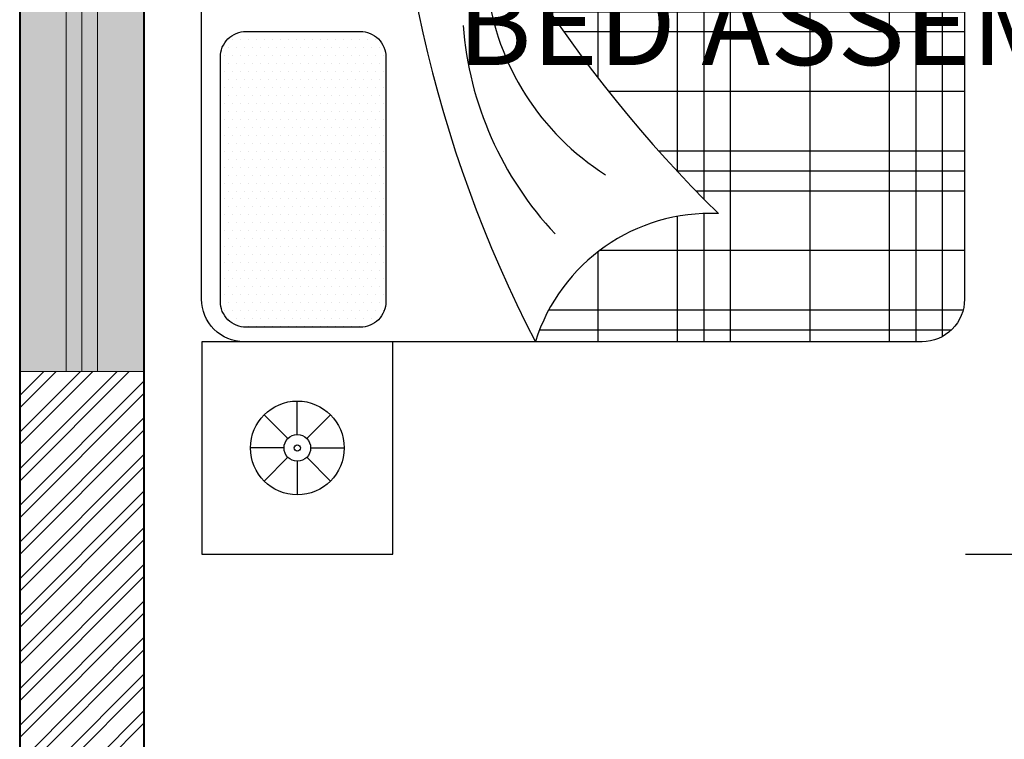
# Model space of a CAD drawing. Units: inches. Extents: x 528 to 2520, y -151 to 1354.
# Tile 4 of 41: x 587 to 658, y 1137 to 1189. Entities that reach past the tile are written whole.
import ezdxf

# ---------------------------------------------------------------- set-up
doc = ezdxf.new("R2010")
doc.units = ezdxf.units.IN
doc.header["$MEASUREMENT"] = 0
for name, color, linetype, lineweight in [('A-ANNO-DIMS', 2, 'Continuous', 18), ('A-FURN', 8, 'Continuous', 18), ('A-WALL-PATT', 6, 'Continuous', 13), ('walls', 7, 'Continuous', 40), ('WINDOWS', 2, 'Continuous', 20)]:
    doc.layers.add(name, color=color, linetype=linetype, lineweight=lineweight)
doc.layers.add('A-GLAZ-PATT', color=152, linetype='Continuous', lineweight=13, true_color=0x2776bb)
doc.layers.add('BLOCK', color=6, linetype='Continuous')
doc.styles.get("Standard").update_dxf_attribs({"font": 'arial.ttf'})
doc.dimstyles.get("Standard").update_dxf_attribs({"dimtxt": 6, "dimasz": 2, "dimexe": 0.18, "dimexo": 0.0625, "dimgap": 0.09, "dimtad": 0, "dimtih": 1, "dimtoh": 1, "dimdec": 1, "dimzin": 0, "dimdsep": 46, "dimlunit": 3, "dimtxsty": 'Standard', "dimblk": 'ARCHTICK', "dimcen": 0.09, "dimadec": 0, "dimazin": 0, "dimtfac": 1, "dimtdec": 1, "dimtofl": 0, "dimtmove": 0, "dimatfit": 3, "dimfxl": 1, "dimtolj": 1, "dimtzin": 0, "dimarcsym": 0})

# ---------------------------------------------------------------- blocks, each defined once
blk = doc.blocks.new('*X15')
at = {"color": 0}
for p, q in [((276.598, 451.25), (280.51, 451.25)), ((275.455, 450.625), (280.51, 450.625)), ((274.411, 450), (280.51, 450)), ((265.51, 448.125), (267.634, 448.125)), ((271.723, 448.125), (280.51, 448.125)), ((265.51, 446.25), (268.465, 446.25)), ((269.519, 446.25), (280.51, 446.25)), ((265.51, 445.625), (268.531, 445.625)), ((268.866, 445.625), (280.51, 445.625)), ((265.51, 445), (280.51, 445)), ((265.51, 443.125), (280.51, 443.125)), ((265.51, 441.25), (280.51, 441.25)), ((265.51, 440.625), (280.51, 440.625)), ((265.634, 440), (280.386, 440))]:
    blk.add_line(p, q, dxfattribs=at)
blk = doc.blocks.new('*X16')
at = {"color": 0}
for p, q in [((280.312, 439.886), (280.312, 452.896)), ((278.906, 439.482), (278.906, 452.338)), ((277.5, 439.482), (277.5, 451.702)), ((277.031, 439.482), (277.031, 451.471)), ((276.562, 439.482), (276.562, 451.231)), ((275.156, 439.482), (275.156, 450.451)), ((265.781, 439.797), (265.781, 449.511)), ((273.75, 439.482), (273.75, 449.576)), ((266.25, 439.517), (266.25, 449.296)), ((273.281, 439.482), (273.281, 449.261)), ((272.812, 439.482), (272.812, 448.934)), ((267.656, 439.482), (267.656, 448.095)), ((271.406, 439.482), (271.406, 447.876)), ((270, 439.482), (270, 446.689)), ((269.531, 439.482), (269.531, 446.262)), ((269.062, 439.482), (269.062, 445.817))]:
    blk.add_line(p, q, dxfattribs=at)
blk = doc.blocks.new('*X17')
at = {"color": 0}
for p, q in [((266.4375, 457.03125), (266.4375, 457.03125)), ((266.8125, 457.03125), (266.8125, 457.03125)), ((267.1875, 457.03125), (267.1875, 457.03125)), ((267.5625, 457.03125), (267.5625, 457.03125)), ((267.9375, 457.03125), (267.9375, 457.03125)), ((268.3125, 457.03125), (268.3125, 457.03125)), ((268.6875, 457.03125), (268.6875, 457.03125)), ((269.0625, 457.03125), (269.0625, 457.03125)), ((269.4375, 457.03125), (269.4375, 457.03125)), ((269.8125, 457.03125), (269.8125, 457.03125)), ((270.1875, 457.03125), (270.1875, 457.03125)), ((270.5625, 457.03125), (270.5625, 457.03125)), ((270.9375, 457.03125), (270.9375, 457.03125)), ((271.3125, 457.03125), (271.3125, 457.03125)), ((271.6875, 457.03125), (271.6875, 457.03125)), ((272.0625, 457.03125), (272.0625, 457.03125)), ((266.0625, 456.84375), (266.0625, 456.84375)), ((266.25, 456.9375), (266.25, 456.9375)), ((266.25, 456.75), (266.25, 456.75)), ((266.4375, 456.84375), (266.4375, 456.84375)), ((266.625, 456.9375), (266.625, 456.9375)), ((266.625, 456.75), (266.625, 456.75)), ((266.8125, 456.84375), (266.8125, 456.84375)), ((267, 456.9375), (267, 456.9375)), ((267, 456.75), (267, 456.75)), ((267.1875, 456.84375), (267.1875, 456.84375)), ((267.375, 456.9375), (267.375, 456.9375)), ((267.375, 456.75), (267.375, 456.75)), ((267.5625, 456.84375), (267.5625, 456.84375)), ((267.75, 456.9375), (267.75, 456.9375)), ((267.75, 456.75), (267.75, 456.75)), ((267.9375, 456.84375), (267.9375, 456.84375)), ((268.125, 456.9375), (268.125, 456.9375)), ((268.125, 456.75), (268.125, 456.75)), ((268.3125, 456.84375), (268.3125, 456.84375)), ((268.5, 456.9375), (268.5, 456.9375)), ((268.5, 456.75), (268.5, 456.75)), ((268.6875, 456.84375), (268.6875, 456.84375)), ((268.875, 456.9375), (268.875, 456.9375)), ((268.875, 456.75), (268.875, 456.75)), ((269.0625, 456.84375), (269.0625, 456.84375)), ((269.25, 456.9375), (269.25, 456.9375)), ((269.25, 456.75), (269.25, 456.75)), ((269.4375, 456.84375), (269.4375, 456.84375)), ((269.625, 456.9375), (269.625, 456.9375)), ((269.625, 456.75), (269.625, 456.75)), ((269.8125, 456.84375), (269.8125, 456.84375)), ((270, 456.9375), (270, 456.9375)), ((270, 456.75), (270, 456.75)), ((270.1875, 456.84375), (270.1875, 456.84375)), ((270.375, 456.9375), (270.375, 456.9375)), ((270.375, 456.75), (270.375, 456.75)), ((270.5625, 456.84375), (270.5625, 456.84375)), ((270.75, 456.9375), (270.75, 456.9375)), ((270.75, 456.75), (270.75, 456.75)), ((270.9375, 456.84375), (270.9375, 456.84375)), ((271.125, 456.9375), (271.125, 456.9375)), ((271.125, 456.75), (271.125, 456.75)), ((271.3125, 456.84375), (271.3125, 456.84375)), ((271.5, 456.9375), (271.5, 456.9375)), ((271.5, 456.75), (271.5, 456.75)), ((271.6875, 456.84375), (271.6875, 456.84375)), ((271.875, 456.9375), (271.875, 456.9375)), ((271.875, 456.75), (271.875, 456.75)), ((272.0625, 456.84375), (272.0625, 456.84375)), ((272.25, 456.9375), (272.25, 456.9375)), ((272.25, 456.75), (272.25, 456.75)), ((272.4375, 456.84375), (272.4375, 456.84375)), ((272.625, 456.75), (272.625, 456.75)), ((265.875, 456.5625), (265.875, 456.5625)), ((266.0625, 456.65625), (266.0625, 456.65625)), ((266.25, 456.5625), (266.25, 456.5625)), ((266.4375, 456.65625), (266.4375, 456.65625)), ((266.625, 456.5625), (266.625, 456.5625)), ((266.8125, 456.65625), (266.8125, 456.65625)), ((267, 456.5625), (267, 456.5625)), ((267.1875, 456.65625), (267.1875, 456.65625)), ((267.375, 456.5625), (267.375, 456.5625)), ((267.5625, 456.65625), (267.5625, 456.65625)), ((267.75, 456.5625), (267.75, 456.5625)), ((267.9375, 456.65625), (267.9375, 456.65625)), ((268.125, 456.5625), (268.125, 456.5625)), ((268.3125, 456.65625), (268.3125, 456.65625)), ((268.5, 456.5625), (268.5, 456.5625)), ((268.6875, 456.65625), (268.6875, 456.65625)), ((268.875, 456.5625), (268.875, 456.5625)), ((269.0625, 456.65625), (269.0625, 456.65625)), ((269.25, 456.5625), (269.25, 456.5625)), ((269.4375, 456.65625), (269.4375, 456.65625)), ((269.625, 456.5625), (269.625, 456.5625)), ((269.8125, 456.65625), (269.8125, 456.65625)), ((270, 456.5625), (270, 456.5625)), ((270.1875, 456.65625), (270.1875, 456.65625)), ((270.375, 456.5625), (270.375, 456.5625)), ((270.5625, 456.65625), (270.5625, 456.65625)), ((270.75, 456.5625), (270.75, 456.5625)), ((270.9375, 456.65625), (270.9375, 456.65625)), ((271.125, 456.5625), (271.125, 456.5625)), ((271.3125, 456.65625), (271.3125, 456.65625)), ((271.5, 456.5625), (271.5, 456.5625)), ((271.6875, 456.65625), (271.6875, 456.65625)), ((271.875, 456.5625), (271.875, 456.5625)), ((272.0625, 456.65625), (272.0625, 456.65625)), ((272.25, 456.5625), (272.25, 456.5625)), ((272.4375, 456.65625), (272.4375, 456.65625)), ((272.625, 456.5625), (272.625, 456.5625)), ((265.875, 456.375), (265.875, 456.375)), ((266.0625, 456.46875), (266.0625, 456.46875)), ((266.0625, 456.28125), (266.0625, 456.28125)), ((266.25, 456.375), (266.25, 456.375)), ((266.4375, 456.46875), (266.4375, 456.46875)), ((266.4375, 456.28125), (266.4375, 456.28125)), ((266.625, 456.375), (266.625, 456.375)), ((266.8125, 456.46875), (266.8125, 456.46875)), ((266.8125, 456.28125), (266.8125, 456.28125)), ((267, 456.375), (267, 456.375)), ((267.1875, 456.46875), (267.1875, 456.46875)), ((267.1875, 456.28125), (267.1875, 456.28125)), ((267.375, 456.375), (267.375, 456.375)), ((267.5625, 456.46875), (267.5625, 456.46875)), ((267.5625, 456.28125), (267.5625, 456.28125)), ((267.75, 456.375), (267.75, 456.375)), ((267.9375, 456.46875), (267.9375, 456.46875)), ((267.9375, 456.28125), (267.9375, 456.28125)), ((268.125, 456.375), (268.125, 456.375)), ((268.3125, 456.46875), (268.3125, 456.46875)), ((268.3125, 456.28125), (268.3125, 456.28125)), ((268.5, 456.375), (268.5, 456.375)), ((268.6875, 456.46875), (268.6875, 456.46875)), ((268.6875, 456.28125), (268.6875, 456.28125)), ((268.875, 456.375), (268.875, 456.375)), ((269.0625, 456.46875), (269.0625, 456.46875)), ((269.0625, 456.28125), (269.0625, 456.28125)), ((269.25, 456.375), (269.25, 456.375)), ((269.4375, 456.46875), (269.4375, 456.46875)), ((269.4375, 456.28125), (269.4375, 456.28125)), ((269.625, 456.375), (269.625, 456.375)), ((269.8125, 456.46875), (269.8125, 456.46875)), ((269.8125, 456.28125), (269.8125, 456.28125)), ((270, 456.375), (270, 456.375)), ((270.1875, 456.46875), (270.1875, 456.46875)), ((270.1875, 456.28125), (270.1875, 456.28125)), ((270.375, 456.375), (270.375, 456.375)), ((270.5625, 456.46875), (270.5625, 456.46875)), ((270.5625, 456.28125), (270.5625, 456.28125)), ((270.75, 456.375), (270.75, 456.375)), ((270.9375, 456.46875), (270.9375, 456.46875)), ((270.9375, 456.28125), (270.9375, 456.28125)), ((271.125, 456.375), (271.125, 456.375)), ((271.3125, 456.46875), (271.3125, 456.46875)), ((271.3125, 456.28125), (271.3125, 456.28125)), ((271.5, 456.375), (271.5, 456.375)), ((271.6875, 456.46875), (271.6875, 456.46875)), ((271.6875, 456.28125), (271.6875, 456.28125)), ((271.875, 456.375), (271.875, 456.375)), ((272.0625, 456.46875), (272.0625, 456.46875)), ((272.0625, 456.28125), (272.0625, 456.28125)), ((272.25, 456.375), (272.25, 456.375)), ((272.4375, 456.46875), (272.4375, 456.46875)), ((272.4375, 456.28125), (272.4375, 456.28125)), ((272.625, 456.375), (272.625, 456.375)), ((272.8125, 456.46875), (272.8125, 456.46875)), ((272.8125, 456.28125), (272.8125, 456.28125)), ((265.875, 456.1875), (265.875, 456.1875)), ((266.0625, 456.09375), (266.0625, 456.09375)), ((266.25, 456.1875), (266.25, 456.1875)), ((266.4375, 456.09375), (266.4375, 456.09375)), ((266.625, 456.1875), (266.625, 456.1875)), ((266.8125, 456.09375), (266.8125, 456.09375)), ((267, 456.1875), (267, 456.1875)), ((267.1875, 456.09375), (267.1875, 456.09375)), ((267.375, 456.1875), (267.375, 456.1875)), ((267.5625, 456.09375), (267.5625, 456.09375)), ((267.75, 456.1875), (267.75, 456.1875)), ((267.9375, 456.09375), (267.9375, 456.09375)), ((268.125, 456.1875), (268.125, 456.1875)), ((268.3125, 456.09375), (268.3125, 456.09375)), ((268.5, 456.1875), (268.5, 456.1875)), ((268.6875, 456.09375), (268.6875, 456.09375)), ((268.875, 456.1875), (268.875, 456.1875)), ((269.0625, 456.09375), (269.0625, 456.09375)), ((269.25, 456.1875), (269.25, 456.1875)), ((269.4375, 456.09375), (269.4375, 456.09375)), ((269.625, 456.1875), (269.625, 456.1875)), ((269.8125, 456.09375), (269.8125, 456.09375)), ((270, 456.1875), (270, 456.1875)), ((270.1875, 456.09375), (270.1875, 456.09375)), ((270.375, 456.1875), (270.375, 456.1875)), ((270.5625, 456.09375), (270.5625, 456.09375)), ((270.75, 456.1875), (270.75, 456.1875)), ((270.9375, 456.09375), (270.9375, 456.09375)), ((271.125, 456.1875), (271.125, 456.1875)), ((271.3125, 456.09375), (271.3125, 456.09375)), ((271.5, 456.1875), (271.5, 456.1875)), ((271.6875, 456.09375), (271.6875, 456.09375)), ((271.875, 456.1875), (271.875, 456.1875)), ((272.0625, 456.09375), (272.0625, 456.09375)), ((272.25, 456.1875), (272.25, 456.1875)), ((272.4375, 456.09375), (272.4375, 456.09375)), ((272.625, 456.1875), (272.625, 456.1875)), ((272.8125, 456.09375), (272.8125, 456.09375)), ((265.875, 456), (265.875, 456)), ((265.875, 455.8125), (265.875, 455.8125)), ((266.0625, 455.90625), (266.0625, 455.90625)), ((266.25, 456), (266.25, 456)), ((266.25, 455.8125), (266.25, 455.8125)), ((266.4375, 455.90625), (266.4375, 455.90625)), ((266.625, 456), (266.625, 456)), ((266.625, 455.8125), (266.625, 455.8125)), ((266.8125, 455.90625), (266.8125, 455.90625)), ((267, 456), (267, 456)), ((267, 455.8125), (267, 455.8125)), ((267.1875, 455.90625), (267.1875, 455.90625)), ((267.375, 456), (267.375, 456)), ((267.375, 455.8125), (267.375, 455.8125)), ((267.5625, 455.90625), (267.5625, 455.90625)), ((267.75, 456), (267.75, 456)), ((267.75, 455.8125), (267.75, 455.8125)), ((267.9375, 455.90625), (267.9375, 455.90625)), ((268.125, 456), (268.125, 456)), ((268.125, 455.8125), (268.125, 455.8125)), ((268.3125, 455.90625), (268.3125, 455.90625)), ((268.5, 456), (268.5, 456)), ((268.5, 455.8125), (268.5, 455.8125)), ((268.6875, 455.90625), (268.6875, 455.90625)), ((268.875, 456), (268.875, 456)), ((268.875, 455.8125), (268.875, 455.8125)), ((269.0625, 455.90625), (269.0625, 455.90625)), ((269.25, 456), (269.25, 456)), ((269.25, 455.8125), (269.25, 455.8125)), ((269.4375, 455.90625), (269.4375, 455.90625)), ((269.625, 456), (269.625, 456)), ((269.625, 455.8125), (269.625, 455.8125)), ((269.8125, 455.90625), (269.8125, 455.90625)), ((270, 456), (270, 456)), ((270, 455.8125), (270, 455.8125)), ((270.1875, 455.90625), (270.1875, 455.90625)), ((270.375, 456), (270.375, 456)), ((270.375, 455.8125), (270.375, 455.8125)), ((270.5625, 455.90625), (270.5625, 455.90625)), ((270.75, 456), (270.75, 456)), ((270.75, 455.8125), (270.75, 455.8125)), ((270.9375, 455.90625), (270.9375, 455.90625)), ((271.125, 456), (271.125, 456)), ((271.125, 455.8125), (271.125, 455.8125)), ((271.3125, 455.90625), (271.3125, 455.90625)), ((271.5, 456), (271.5, 456)), ((271.5, 455.8125), (271.5, 455.8125)), ((271.6875, 455.90625), (271.6875, 455.90625)), ((271.875, 456), (271.875, 456)), ((271.875, 455.8125), (271.875, 455.8125)), ((272.0625, 455.90625), (272.0625, 455.90625)), ((272.25, 456), (272.25, 456)), ((272.25, 455.8125), (272.25, 455.8125)), ((272.4375, 455.90625), (272.4375, 455.90625)), ((272.625, 456), (272.625, 456)), ((272.625, 455.8125), (272.625, 455.8125)), ((272.8125, 455.90625), (272.8125, 455.90625)), ((265.875, 455.625), (265.875, 455.625)), ((266.0625, 455.71875), (266.0625, 455.71875)), ((266.25, 455.625), (266.25, 455.625)), ((266.4375, 455.71875), (266.4375, 455.71875)), ((266.625, 455.625), (266.625, 455.625)), ((266.8125, 455.71875), (266.8125, 455.71875)), ((267, 455.625), (267, 455.625)), ((267.1875, 455.71875), (267.1875, 455.71875)), ((267.375, 455.625), (267.375, 455.625)), ((267.5625, 455.71875), (267.5625, 455.71875)), ((267.75, 455.625), (267.75, 455.625)), ((267.9375, 455.71875), (267.9375, 455.71875)), ((268.125, 455.625), (268.125, 455.625)), ((268.3125, 455.71875), (268.3125, 455.71875)), ((268.5, 455.625), (268.5, 455.625)), ((268.6875, 455.71875), (268.6875, 455.71875)), ((268.875, 455.625), (268.875, 455.625)), ((269.0625, 455.71875), (269.0625, 455.71875)), ((269.25, 455.625), (269.25, 455.625)), ((269.4375, 455.71875), (269.4375, 455.71875)), ((269.625, 455.625), (269.625, 455.625)), ((269.8125, 455.71875), (269.8125, 455.71875)), ((270, 455.625), (270, 455.625)), ((270.1875, 455.71875), (270.1875, 455.71875)), ((270.375, 455.625), (270.375, 455.625)), ((270.5625, 455.71875), (270.5625, 455.71875)), ((270.75, 455.625), (270.75, 455.625)), ((270.9375, 455.71875), (270.9375, 455.71875)), ((271.125, 455.625), (271.125, 455.625)), ((271.3125, 455.71875), (271.3125, 455.71875)), ((271.5, 455.625), (271.5, 455.625)), ((271.6875, 455.71875), (271.6875, 455.71875)), ((271.875, 455.625), (271.875, 455.625)), ((272.0625, 455.71875), (272.0625, 455.71875)), ((272.25, 455.625), (272.25, 455.625)), ((272.4375, 455.71875), (272.4375, 455.71875)), ((272.625, 455.625), (272.625, 455.625)), ((272.8125, 455.71875), (272.8125, 455.71875)), ((265.875, 455.4375), (265.875, 455.4375)), ((266.0625, 455.53125), (266.0625, 455.53125)), ((266.0625, 455.34375), (266.0625, 455.34375)), ((266.25, 455.4375), (266.25, 455.4375)), ((266.4375, 455.53125), (266.4375, 455.53125)), ((266.4375, 455.34375), (266.4375, 455.34375)), ((266.625, 455.4375), (266.625, 455.4375)), ((266.8125, 455.53125), (266.8125, 455.53125)), ((266.8125, 455.34375), (266.8125, 455.34375)), ((267, 455.4375), (267, 455.4375)), ((267.1875, 455.53125), (267.1875, 455.53125)), ((267.1875, 455.34375), (267.1875, 455.34375)), ((267.375, 455.4375), (267.375, 455.4375)), ((267.5625, 455.53125), (267.5625, 455.53125)), ((267.5625, 455.34375), (267.5625, 455.34375)), ((267.75, 455.4375), (267.75, 455.4375)), ((267.9375, 455.53125), (267.9375, 455.53125)), ((267.9375, 455.34375), (267.9375, 455.34375)), ((268.125, 455.4375), (268.125, 455.4375)), ((268.3125, 455.53125), (268.3125, 455.53125)), ((268.3125, 455.34375), (268.3125, 455.34375)), ((268.5, 455.4375), (268.5, 455.4375)), ((268.6875, 455.53125), (268.6875, 455.53125)), ((268.6875, 455.34375), (268.6875, 455.34375)), ((268.875, 455.4375), (268.875, 455.4375)), ((269.0625, 455.53125), (269.0625, 455.53125)), ((269.0625, 455.34375), (269.0625, 455.34375)), ((269.25, 455.4375), (269.25, 455.4375)), ((269.4375, 455.53125), (269.4375, 455.53125)), ((269.4375, 455.34375), (269.4375, 455.34375)), ((269.625, 455.4375), (269.625, 455.4375)), ((269.8125, 455.53125), (269.8125, 455.53125)), ((269.8125, 455.34375), (269.8125, 455.34375)), ((270, 455.4375), (270, 455.4375)), ((270.1875, 455.53125), (270.1875, 455.53125)), ((270.1875, 455.34375), (270.1875, 455.34375)), ((270.375, 455.4375), (270.375, 455.4375)), ((270.5625, 455.53125), (270.5625, 455.53125)), ((270.5625, 455.34375), (270.5625, 455.34375)), ((270.75, 455.4375), (270.75, 455.4375)), ((270.9375, 455.53125), (270.9375, 455.53125)), ((270.9375, 455.34375), (270.9375, 455.34375)), ((271.125, 455.4375), (271.125, 455.4375)), ((271.3125, 455.53125), (271.3125, 455.53125)), ((271.3125, 455.34375), (271.3125, 455.34375)), ((271.5, 455.4375), (271.5, 455.4375)), ((271.6875, 455.53125), (271.6875, 455.53125)), ((271.6875, 455.34375), (271.6875, 455.34375)), ((271.875, 455.4375), (271.875, 455.4375)), ((272.0625, 455.53125), (272.0625, 455.53125)), ((272.0625, 455.34375), (272.0625, 455.34375)), ((272.25, 455.4375), (272.25, 455.4375)), ((272.4375, 455.53125), (272.4375, 455.53125)), ((272.4375, 455.34375), (272.4375, 455.34375)), ((272.625, 455.4375), (272.625, 455.4375)), ((272.8125, 455.53125), (272.8125, 455.53125)), ((272.8125, 455.34375), (272.8125, 455.34375)), ((265.875, 455.25), (265.875, 455.25)), ((266.0625, 455.15625), (266.0625, 455.15625)), ((266.25, 455.25), (266.25, 455.25)), ((266.4375, 455.15625), (266.4375, 455.15625)), ((266.625, 455.25), (266.625, 455.25)), ((266.8125, 455.15625), (266.8125, 455.15625)), ((267, 455.25), (267, 455.25)), ((267.1875, 455.15625), (267.1875, 455.15625)), ((267.375, 455.25), (267.375, 455.25)), ((267.5625, 455.15625), (267.5625, 455.15625)), ((267.75, 455.25), (267.75, 455.25)), ((267.9375, 455.15625), (267.9375, 455.15625)), ((268.125, 455.25), (268.125, 455.25)), ((268.3125, 455.15625), (268.3125, 455.15625)), ((268.5, 455.25), (268.5, 455.25)), ((268.6875, 455.15625), (268.6875, 455.15625)), ((268.875, 455.25), (268.875, 455.25)), ((269.0625, 455.15625), (269.0625, 455.15625)), ((269.25, 455.25), (269.25, 455.25)), ((269.4375, 455.15625), (269.4375, 455.15625)), ((269.625, 455.25), (269.625, 455.25)), ((269.8125, 455.15625), (269.8125, 455.15625)), ((270, 455.25), (270, 455.25)), ((270.1875, 455.15625), (270.1875, 455.15625)), ((270.375, 455.25), (270.375, 455.25)), ((270.5625, 455.15625), (270.5625, 455.15625)), ((270.75, 455.25), (270.75, 455.25)), ((270.9375, 455.15625), (270.9375, 455.15625)), ((271.125, 455.25), (271.125, 455.25)), ((271.3125, 455.15625), (271.3125, 455.15625)), ((271.5, 455.25), (271.5, 455.25)), ((271.6875, 455.15625), (271.6875, 455.15625)), ((271.875, 455.25), (271.875, 455.25)), ((272.0625, 455.15625), (272.0625, 455.15625)), ((272.25, 455.25), (272.25, 455.25)), ((272.4375, 455.15625), (272.4375, 455.15625)), ((272.625, 455.25), (272.625, 455.25)), ((272.8125, 455.15625), (272.8125, 455.15625)), ((265.875, 455.0625), (265.875, 455.0625)), ((265.875, 454.875), (265.875, 454.875)), ((266.0625, 454.96875), (266.0625, 454.96875)), ((266.25, 455.0625), (266.25, 455.0625)), ((266.25, 454.875), (266.25, 454.875)), ((266.4375, 454.96875), (266.4375, 454.96875)), ((266.625, 455.0625), (266.625, 455.0625)), ((266.625, 454.875), (266.625, 454.875)), ((266.8125, 454.96875), (266.8125, 454.96875)), ((267, 455.0625), (267, 455.0625)), ((267, 454.875), (267, 454.875)), ((267.1875, 454.96875), (267.1875, 454.96875)), ((267.375, 455.0625), (267.375, 455.0625)), ((267.375, 454.875), (267.375, 454.875)), ((267.5625, 454.96875), (267.5625, 454.96875)), ((267.75, 455.0625), (267.75, 455.0625)), ((267.75, 454.875), (267.75, 454.875)), ((267.9375, 454.96875), (267.9375, 454.96875)), ((268.125, 455.0625), (268.125, 455.0625)), ((268.125, 454.875), (268.125, 454.875)), ((268.3125, 454.96875), (268.3125, 454.96875)), ((268.5, 455.0625), (268.5, 455.0625)), ((268.5, 454.875), (268.5, 454.875)), ((268.6875, 454.96875), (268.6875, 454.96875)), ((268.875, 455.0625), (268.875, 455.0625)), ((268.875, 454.875), (268.875, 454.875)), ((269.0625, 454.96875), (269.0625, 454.96875)), ((269.25, 455.0625), (269.25, 455.0625)), ((269.25, 454.875), (269.25, 454.875)), ((269.4375, 454.96875), (269.4375, 454.96875)), ((269.625, 455.0625), (269.625, 455.0625)), ((269.625, 454.875), (269.625, 454.875)), ((269.8125, 454.96875), (269.8125, 454.96875)), ((270, 455.0625), (270, 455.0625)), ((270, 454.875), (270, 454.875)), ((270.1875, 454.96875), (270.1875, 454.96875)), ((270.375, 455.0625), (270.375, 455.0625)), ((270.375, 454.875), (270.375, 454.875)), ((270.5625, 454.96875), (270.5625, 454.96875)), ((270.75, 455.0625), (270.75, 455.0625)), ((270.75, 454.875), (270.75, 454.875)), ((270.9375, 454.96875), (270.9375, 454.96875)), ((271.125, 455.0625), (271.125, 455.0625)), ((271.125, 454.875), (271.125, 454.875)), ((271.3125, 454.96875), (271.3125, 454.96875)), ((271.5, 455.0625), (271.5, 455.0625)), ((271.5, 454.875), (271.5, 454.875)), ((271.6875, 454.96875), (271.6875, 454.96875)), ((271.875, 455.0625), (271.875, 455.0625)), ((271.875, 454.875), (271.875, 454.875)), ((272.0625, 454.96875), (272.0625, 454.96875)), ((272.25, 455.0625), (272.25, 455.0625)), ((272.25, 454.875), (272.25, 454.875)), ((272.4375, 454.96875), (272.4375, 454.96875)), ((272.625, 455.0625), (272.625, 455.0625)), ((272.625, 454.875), (272.625, 454.875)), ((272.8125, 454.96875), (272.8125, 454.96875)), ((265.875, 454.6875), (265.875, 454.6875)), ((266.0625, 454.78125), (266.0625, 454.78125)), ((266.25, 454.6875), (266.25, 454.6875)), ((266.4375, 454.78125), (266.4375, 454.78125)), ((266.625, 454.6875), (266.625, 454.6875)), ((266.8125, 454.78125), (266.8125, 454.78125)), ((267, 454.6875), (267, 454.6875)), ((267.1875, 454.78125), (267.1875, 454.78125)), ((267.375, 454.6875), (267.375, 454.6875)), ((267.5625, 454.78125), (267.5625, 454.78125)), ((267.75, 454.6875), (267.75, 454.6875)), ((267.9375, 454.78125), (267.9375, 454.78125)), ((268.125, 454.6875), (268.125, 454.6875)), ((268.3125, 454.78125), (268.3125, 454.78125)), ((268.5, 454.6875), (268.5, 454.6875)), ((268.6875, 454.78125), (268.6875, 454.78125)), ((268.875, 454.6875), (268.875, 454.6875)), ((269.0625, 454.78125), (269.0625, 454.78125)), ((269.25, 454.6875), (269.25, 454.6875)), ((269.4375, 454.78125), (269.4375, 454.78125)), ((269.625, 454.6875), (269.625, 454.6875)), ((269.8125, 454.78125), (269.8125, 454.78125)), ((270, 454.6875), (270, 454.6875)), ((270.1875, 454.78125), (270.1875, 454.78125)), ((270.375, 454.6875), (270.375, 454.6875)), ((270.5625, 454.78125), (270.5625, 454.78125)), ((270.75, 454.6875), (270.75, 454.6875)), ((270.9375, 454.78125), (270.9375, 454.78125)), ((271.125, 454.6875), (271.125, 454.6875)), ((271.3125, 454.78125), (271.3125, 454.78125)), ((271.5, 454.6875), (271.5, 454.6875)), ((271.6875, 454.78125), (271.6875, 454.78125)), ((271.875, 454.6875), (271.875, 454.6875)), ((272.0625, 454.78125), (272.0625, 454.78125)), ((272.25, 454.6875), (272.25, 454.6875)), ((272.4375, 454.78125), (272.4375, 454.78125)), ((272.625, 454.6875), (272.625, 454.6875)), ((272.8125, 454.78125), (272.8125, 454.78125)), ((265.875, 454.5), (265.875, 454.5)), ((266.0625, 454.59375), (266.0625, 454.59375)), ((266.0625, 454.40625), (266.0625, 454.40625)), ((266.25, 454.5), (266.25, 454.5)), ((266.4375, 454.59375), (266.4375, 454.59375)), ((266.4375, 454.40625), (266.4375, 454.40625)), ((266.625, 454.5), (266.625, 454.5)), ((266.8125, 454.59375), (266.8125, 454.59375)), ((266.8125, 454.40625), (266.8125, 454.40625)), ((267, 454.5), (267, 454.5)), ((267.1875, 454.59375), (267.1875, 454.59375)), ((267.1875, 454.40625), (267.1875, 454.40625)), ((267.375, 454.5), (267.375, 454.5)), ((267.5625, 454.59375), (267.5625, 454.59375)), ((267.5625, 454.40625), (267.5625, 454.40625)), ((267.75, 454.5), (267.75, 454.5)), ((267.9375, 454.59375), (267.9375, 454.59375)), ((267.9375, 454.40625), (267.9375, 454.40625)), ((268.125, 454.5), (268.125, 454.5)), ((268.3125, 454.59375), (268.3125, 454.59375)), ((268.3125, 454.40625), (268.3125, 454.40625)), ((268.5, 454.5), (268.5, 454.5)), ((268.6875, 454.59375), (268.6875, 454.59375)), ((268.6875, 454.40625), (268.6875, 454.40625)), ((268.875, 454.5), (268.875, 454.5)), ((269.0625, 454.59375), (269.0625, 454.59375)), ((269.0625, 454.40625), (269.0625, 454.40625)), ((269.25, 454.5), (269.25, 454.5)), ((269.4375, 454.59375), (269.4375, 454.59375)), ((269.4375, 454.40625), (269.4375, 454.40625)), ((269.625, 454.5), (269.625, 454.5)), ((269.8125, 454.59375), (269.8125, 454.59375)), ((269.8125, 454.40625), (269.8125, 454.40625)), ((270, 454.5), (270, 454.5)), ((270.1875, 454.59375), (270.1875, 454.59375)), ((270.1875, 454.40625), (270.1875, 454.40625)), ((270.375, 454.5), (270.375, 454.5)), ((270.5625, 454.59375), (270.5625, 454.59375)), ((270.5625, 454.40625), (270.5625, 454.40625)), ((270.75, 454.5), (270.75, 454.5)), ((270.9375, 454.59375), (270.9375, 454.59375)), ((270.9375, 454.40625), (270.9375, 454.40625)), ((271.125, 454.5), (271.125, 454.5)), ((271.3125, 454.59375), (271.3125, 454.59375)), ((271.3125, 454.40625), (271.3125, 454.40625)), ((271.5, 454.5), (271.5, 454.5)), ((271.6875, 454.59375), (271.6875, 454.59375)), ((271.6875, 454.40625), (271.6875, 454.40625)), ((271.875, 454.5), (271.875, 454.5)), ((272.0625, 454.59375), (272.0625, 454.59375)), ((272.0625, 454.40625), (272.0625, 454.40625)), ((272.25, 454.5), (272.25, 454.5)), ((272.4375, 454.59375), (272.4375, 454.59375)), ((272.4375, 454.40625), (272.4375, 454.40625)), ((272.625, 454.5), (272.625, 454.5)), ((272.8125, 454.59375), (272.8125, 454.59375)), ((272.8125, 454.40625), (272.8125, 454.40625)), ((265.875, 454.3125), (265.875, 454.3125)), ((266.0625, 454.21875), (266.0625, 454.21875)), ((266.25, 454.3125), (266.25, 454.3125)), ((266.4375, 454.21875), (266.4375, 454.21875)), ((266.625, 454.3125), (266.625, 454.3125)), ((266.8125, 454.21875), (266.8125, 454.21875)), ((267, 454.3125), (267, 454.3125)), ((267.1875, 454.21875), (267.1875, 454.21875)), ((267.375, 454.3125), (267.375, 454.3125)), ((267.5625, 454.21875), (267.5625, 454.21875)), ((267.75, 454.3125), (267.75, 454.3125)), ((267.9375, 454.21875), (267.9375, 454.21875)), ((268.125, 454.3125), (268.125, 454.3125)), ((268.3125, 454.21875), (268.3125, 454.21875)), ((268.5, 454.3125), (268.5, 454.3125)), ((268.6875, 454.21875), (268.6875, 454.21875)), ((268.875, 454.3125), (268.875, 454.3125)), ((269.0625, 454.21875), (269.0625, 454.21875)), ((269.25, 454.3125), (269.25, 454.3125)), ((269.4375, 454.21875), (269.4375, 454.21875)), ((269.625, 454.3125), (269.625, 454.3125)), ((269.8125, 454.21875), (269.8125, 454.21875)), ((270, 454.3125), (270, 454.3125)), ((270.1875, 454.21875), (270.1875, 454.21875)), ((270.375, 454.3125), (270.375, 454.3125)), ((270.5625, 454.21875), (270.5625, 454.21875)), ((270.75, 454.3125), (270.75, 454.3125)), ((270.9375, 454.21875), (270.9375, 454.21875)), ((271.125, 454.3125), (271.125, 454.3125)), ((271.3125, 454.21875), (271.3125, 454.21875)), ((271.5, 454.3125), (271.5, 454.3125)), ((271.6875, 454.21875), (271.6875, 454.21875)), ((271.875, 454.3125), (271.875, 454.3125)), ((272.0625, 454.21875), (272.0625, 454.21875)), ((272.25, 454.3125), (272.25, 454.3125)), ((272.4375, 454.21875), (272.4375, 454.21875)), ((272.625, 454.3125), (272.625, 454.3125)), ((272.8125, 454.21875), (272.8125, 454.21875)), ((265.875, 454.125), (265.875, 454.125)), ((265.875, 453.9375), (265.875, 453.9375)), ((266.0625, 454.03125), (266.0625, 454.03125)), ((266.25, 454.125), (266.25, 454.125)), ((266.25, 453.9375), (266.25, 453.9375)), ((266.4375, 454.03125), (266.4375, 454.03125)), ((266.625, 454.125), (266.625, 454.125)), ((266.625, 453.9375), (266.625, 453.9375)), ((266.8125, 454.03125), (266.8125, 454.03125)), ((267, 454.125), (267, 454.125)), ((267, 453.9375), (267, 453.9375)), ((267.1875, 454.03125), (267.1875, 454.03125)), ((267.375, 454.125), (267.375, 454.125)), ((267.375, 453.9375), (267.375, 453.9375)), ((267.5625, 454.03125), (267.5625, 454.03125)), ((267.75, 454.125), (267.75, 454.125)), ((267.75, 453.9375), (267.75, 453.9375)), ((267.9375, 454.03125), (267.9375, 454.03125)), ((268.125, 454.125), (268.125, 454.125)), ((268.125, 453.9375), (268.125, 453.9375)), ((268.3125, 454.03125), (268.3125, 454.03125)), ((268.5, 454.125), (268.5, 454.125)), ((268.5, 453.9375), (268.5, 453.9375)), ((268.6875, 454.03125), (268.6875, 454.03125)), ((268.875, 454.125), (268.875, 454.125)), ((268.875, 453.9375), (268.875, 453.9375)), ((269.0625, 454.03125), (269.0625, 454.03125)), ((269.25, 454.125), (269.25, 454.125)), ((269.25, 453.9375), (269.25, 453.9375)), ((269.4375, 454.03125), (269.4375, 454.03125)), ((269.625, 454.125), (269.625, 454.125)), ((269.625, 453.9375), (269.625, 453.9375)), ((269.8125, 454.03125), (269.8125, 454.03125)), ((270, 454.125), (270, 454.125)), ((270, 453.9375), (270, 453.9375)), ((270.1875, 454.03125), (270.1875, 454.03125)), ((270.375, 454.125), (270.375, 454.125)), ((270.375, 453.9375), (270.375, 453.9375)), ((270.5625, 454.03125), (270.5625, 454.03125)), ((270.75, 454.125), (270.75, 454.125)), ((270.75, 453.9375), (270.75, 453.9375)), ((270.9375, 454.03125), (270.9375, 454.03125)), ((271.125, 454.125), (271.125, 454.125)), ((271.125, 453.9375), (271.125, 453.9375)), ((271.3125, 454.03125), (271.3125, 454.03125)), ((271.5, 454.125), (271.5, 454.125)), ((271.5, 453.9375), (271.5, 453.9375)), ((271.6875, 454.03125), (271.6875, 454.03125)), ((271.875, 454.125), (271.875, 454.125)), ((271.875, 453.9375), (271.875, 453.9375)), ((272.0625, 454.03125), (272.0625, 454.03125)), ((272.25, 454.125), (272.25, 454.125)), ((272.25, 453.9375), (272.25, 453.9375)), ((272.4375, 454.03125), (272.4375, 454.03125)), ((272.625, 454.125), (272.625, 454.125)), ((272.625, 453.9375), (272.625, 453.9375)), ((272.8125, 454.03125), (272.8125, 454.03125)), ((265.875, 453.75), (265.875, 453.75)), ((266.0625, 453.84375), (266.0625, 453.84375)), ((266.25, 453.75), (266.25, 453.75)), ((266.4375, 453.84375), (266.4375, 453.84375)), ((266.625, 453.75), (266.625, 453.75)), ((266.8125, 453.84375), (266.8125, 453.84375)), ((267, 453.75), (267, 453.75)), ((267.1875, 453.84375), (267.1875, 453.84375)), ((267.375, 453.75), (267.375, 453.75)), ((267.5625, 453.84375), (267.5625, 453.84375)), ((267.75, 453.75), (267.75, 453.75)), ((267.9375, 453.84375), (267.9375, 453.84375)), ((268.125, 453.75), (268.125, 453.75)), ((268.3125, 453.84375), (268.3125, 453.84375)), ((268.5, 453.75), (268.5, 453.75)), ((268.6875, 453.84375), (268.6875, 453.84375)), ((268.875, 453.75), (268.875, 453.75)), ((269.0625, 453.84375), (269.0625, 453.84375)), ((269.25, 453.75), (269.25, 453.75)), ((269.4375, 453.84375), (269.4375, 453.84375)), ((269.625, 453.75), (269.625, 453.75)), ((269.8125, 453.84375), (269.8125, 453.84375)), ((270, 453.75), (270, 453.75)), ((270.1875, 453.84375), (270.1875, 453.84375)), ((270.375, 453.75), (270.375, 453.75)), ((270.5625, 453.84375), (270.5625, 453.84375)), ((270.75, 453.75), (270.75, 453.75)), ((270.9375, 453.84375), (270.9375, 453.84375)), ((271.125, 453.75), (271.125, 453.75)), ((271.3125, 453.84375), (271.3125, 453.84375)), ((271.5, 453.75), (271.5, 453.75)), ((271.6875, 453.84375), (271.6875, 453.84375)), ((271.875, 453.75), (271.875, 453.75)), ((272.0625, 453.84375), (272.0625, 453.84375)), ((272.25, 453.75), (272.25, 453.75)), ((272.4375, 453.84375), (272.4375, 453.84375)), ((272.625, 453.75), (272.625, 453.75)), ((272.8125, 453.84375), (272.8125, 453.84375)), ((266.0625, 453.65625), (266.0625, 453.65625)), ((266.0625, 453.46875), (266.0625, 453.46875)), ((266.25, 453.5625), (266.25, 453.5625)), ((266.4375, 453.65625), (266.4375, 453.65625)), ((266.4375, 453.46875), (266.4375, 453.46875)), ((266.625, 453.5625), (266.625, 453.5625)), ((266.8125, 453.65625), (266.8125, 453.65625)), ((266.8125, 453.46875), (266.8125, 453.46875)), ((267, 453.5625), (267, 453.5625)), ((267.1875, 453.65625), (267.1875, 453.65625)), ((267.1875, 453.46875), (267.1875, 453.46875)), ((267.375, 453.5625), (267.375, 453.5625)), ((267.5625, 453.65625), (267.5625, 453.65625)), ((267.5625, 453.46875), (267.5625, 453.46875)), ((267.75, 453.5625), (267.75, 453.5625)), ((267.9375, 453.65625), (267.9375, 453.65625)), ((267.9375, 453.46875), (267.9375, 453.46875)), ((268.125, 453.5625), (268.125, 453.5625)), ((268.3125, 453.65625), (268.3125, 453.65625)), ((268.3125, 453.46875), (268.3125, 453.46875)), ((268.5, 453.5625), (268.5, 453.5625)), ((268.6875, 453.65625), (268.6875, 453.65625)), ((268.6875, 453.46875), (268.6875, 453.46875)), ((268.875, 453.5625), (268.875, 453.5625)), ((269.0625, 453.65625), (269.0625, 453.65625)), ((269.0625, 453.46875), (269.0625, 453.46875)), ((269.25, 453.5625), (269.25, 453.5625)), ((269.4375, 453.65625), (269.4375, 453.65625)), ((269.4375, 453.46875), (269.4375, 453.46875)), ((269.625, 453.5625), (269.625, 453.5625)), ((269.8125, 453.65625), (269.8125, 453.65625)), ((269.8125, 453.46875), (269.8125, 453.46875)), ((270, 453.5625), (270, 453.5625)), ((270.1875, 453.65625), (270.1875, 453.65625)), ((270.1875, 453.46875), (270.1875, 453.46875)), ((270.375, 453.5625), (270.375, 453.5625)), ((270.5625, 453.65625), (270.5625, 453.65625)), ((270.5625, 453.46875), (270.5625, 453.46875)), ((270.75, 453.5625), (270.75, 453.5625)), ((270.9375, 453.65625), (270.9375, 453.65625)), ((270.9375, 453.46875), (270.9375, 453.46875)), ((271.125, 453.5625), (271.125, 453.5625)), ((271.3125, 453.65625), (271.3125, 453.65625)), ((271.3125, 453.46875), (271.3125, 453.46875)), ((271.5, 453.5625), (271.5, 453.5625)), ((271.6875, 453.65625), (271.6875, 453.65625)), ((271.6875, 453.46875), (271.6875, 453.46875)), ((271.875, 453.5625), (271.875, 453.5625)), ((272.0625, 453.65625), (272.0625, 453.65625)), ((272.0625, 453.46875), (272.0625, 453.46875)), ((272.25, 453.5625), (272.25, 453.5625)), ((272.4375, 453.65625), (272.4375, 453.65625)), ((272.4375, 453.46875), (272.4375, 453.46875)), ((272.625, 453.5625), (272.625, 453.5625)), ((272.8125, 453.65625), (272.8125, 453.65625)), ((266.0625, 453.28125), (266.0625, 453.28125)), ((266.25, 453.375), (266.25, 453.375)), ((266.4375, 453.28125), (266.4375, 453.28125)), ((266.625, 453.375), (266.625, 453.375)), ((266.8125, 453.28125), (266.8125, 453.28125)), ((267, 453.375), (267, 453.375)), ((267.1875, 453.28125), (267.1875, 453.28125)), ((267.375, 453.375), (267.375, 453.375)), ((267.5625, 453.28125), (267.5625, 453.28125)), ((267.75, 453.375), (267.75, 453.375)), ((267.9375, 453.28125), (267.9375, 453.28125)), ((268.125, 453.375), (268.125, 453.375)), ((268.3125, 453.28125), (268.3125, 453.28125)), ((268.5, 453.375), (268.5, 453.375)), ((268.6875, 453.28125), (268.6875, 453.28125)), ((268.875, 453.375), (268.875, 453.375)), ((269.0625, 453.28125), (269.0625, 453.28125)), ((269.25, 453.375), (269.25, 453.375)), ((269.4375, 453.28125), (269.4375, 453.28125)), ((269.625, 453.375), (269.625, 453.375)), ((269.8125, 453.28125), (269.8125, 453.28125)), ((270, 453.375), (270, 453.375)), ((270.1875, 453.28125), (270.1875, 453.28125)), ((270.375, 453.375), (270.375, 453.375)), ((270.5625, 453.28125), (270.5625, 453.28125)), ((270.75, 453.375), (270.75, 453.375)), ((270.9375, 453.28125), (270.9375, 453.28125)), ((271.125, 453.375), (271.125, 453.375)), ((271.3125, 453.28125), (271.3125, 453.28125)), ((271.5, 453.375), (271.5, 453.375)), ((271.6875, 453.28125), (271.6875, 453.28125)), ((271.875, 453.375), (271.875, 453.375)), ((272.0625, 453.28125), (272.0625, 453.28125)), ((272.25, 453.375), (272.25, 453.375)), ((272.4375, 453.28125), (272.4375, 453.28125)), ((272.625, 453.375), (272.625, 453.375)), ((266.25, 453.1875), (266.25, 453.1875)), ((266.625, 453.1875), (266.625, 453.1875)), ((267, 453.1875), (267, 453.1875)), ((267.375, 453.1875), (267.375, 453.1875)), ((267.75, 453.1875), (267.75, 453.1875)), ((268.125, 453.1875), (268.125, 453.1875)), ((268.5, 453.1875), (268.5, 453.1875)), ((268.875, 453.1875), (268.875, 453.1875)), ((269.25, 453.1875), (269.25, 453.1875)), ((269.625, 453.1875), (269.625, 453.1875)), ((270, 453.1875), (270, 453.1875)), ((270.375, 453.1875), (270.375, 453.1875)), ((270.75, 453.1875), (270.75, 453.1875)), ((271.125, 453.1875), (271.125, 453.1875)), ((271.5, 453.1875), (271.5, 453.1875)), ((271.875, 453.1875), (271.875, 453.1875)), ((272.25, 453.1875), (272.25, 453.1875))]:
    blk.add_line(p, q, dxfattribs=at)
blk = doc.blocks.new('A$C52E67D0D')
at = {"layer": 'BLOCK'}
for p, q in [((250.5, 1605.5), (250.5, 1684.7)), ((228.3, 1596.3), (172.3, 1652.3)), ((272.7, 1596.3), (328.7, 1652.3)), ((219.1, 1574.1), (139.9, 1574.1)), ((281.9, 1574.1), (361.1, 1574.1)), ((228.3, 1551.9), (172.3, 1495.9)), ((250.5, 1542.8), (250.5, 1463.5)), ((272.7, 1551.9), (328.7, 1495.9))]:
    blk.add_line(p, q, dxfattribs=at)
blk.add_lwpolyline([(501, 1348.6), (501, 1799.6), (0, 1799.6), (0, 1348.6)], close=True, dxfattribs=at)
for points in [[(1901, 0), (601, 0, -0.414214), (501, 100), (501, 1700, -0.414214), (601, 1800), (1901, 1800, -0.414214), (2001, 1700), (2001, 100, -0.414214)], [(1171.8, 1365.1), (595.8, 1365.1, -0.414214), (535, 1425.9), (535, 1694.8, -0.414214), (595.8, 1755.7), (1171.8, 1755.7, -0.414214), (1232.6, 1694.8), (1232.6, 1425.9, -0.414214)]]:
    blk.add_lwpolyline(points, format="xyb", close=True, dxfattribs=at)
for radius in [110.6, 31.4, 7.46]:
    blk.add_circle((250.5, 1574.1), radius, dxfattribs=at)
for centre, radius, start, end in [((1888.6, -1664.5), 3015.3, 87.8642, 117.4001), ((3101, -1685.8), 3227.7, 109.926, 135.3977), ((1308.8, 377.9), 807.6, 94.4436, 133.2788), ((1410.8, 520.2), 610.8, 97.2157, 147.6656), ((371.4, 600.4), 432, 357.3792, 72.5379)]:
    blk.add_arc(centre, radius, start, end, dxfattribs=at)
at = {"layer": 'BLOCK', "xscale": 100, "yscale": 100, "zscale": 100}
for name in ['*X17', '*X16', '*X15']:
    blk.add_blockref(name, (-26050, -43948.2), dxfattribs=at)
blk = doc.blocks.new('WINDOW-48x9-PLAN')
for p, q in [((0, 5.632), (48, 5.632)), ((0, 4.5), (48, 4.5)), ((0, 3.368), (48, 3.368))]:
    blk.add_line(p, q)
blk.add_lwpolyline([(0, 9), (48, 9), (48, 0), (0, 0)], close=True)
blk = doc.blocks.new('_ArchTick')
at = {"color": 0, "linetype": 'ByBlock', "const_width": 0.15}
blk.add_lwpolyline([(-0.5, -0.5), (0.5, 0.5)], dxfattribs=at)
blk = doc.blocks.new('*D46')
at = {"layer": 'A-ANNO-DIMS', "color": 0, "lineweight": -2, "transparency": 16777216}
for p, q in [((655.184, 1227.431), (666.821, 1227.431)), ((666.641, 1227.431), (666.641, 1192.223)), ((666.641, 1150.631), (666.641, 1185.839)), ((655.184, 1150.631), (666.821, 1150.631))]:
    blk.add_line(p, q, dxfattribs=at)
at = {"layer": 'Defpoints', "color": 0, "transparency": 16777216}
for p in [(655.121, 1227.431), (666.641, 1227.431), (655.121, 1150.631)]:
    blk.add_point(p, dxfattribs=at)
at = {"layer": 'A-ANNO-DIMS', "color": 0, "lineweight": -2, "transparency": 16777216, "xscale": 2, "yscale": 2, "zscale": 2}
for p, rotation in [((666.641, 1227.431), 90), ((666.641, 1150.631), 270)]:
    blk.add_blockref('_ArchTick', p, dxfattribs=dict(at, rotation=rotation))
at = {"layer": 'A-ANNO-DIMS', "color": 0, "transparency": 16777216, "insert": (666.641, 1189.031), "char_height": 6, "attachment_point": 5}
blk.add_mtext('\\A1;BED ASSEMBLY 6\'-5" TYP.', dxfattribs=at)

msp = doc.modelspace()

# ---------------------------------------------------------------- hatches: boundary and pattern name
at = {"layer": 'A-GLAZ-PATT'}
h = msp.add_hatch(color=256, dxfattribs=at)
h.dxf.hatch_style = 1
h.paths.add_polyline_path([(586.697, 1211.855), (586.697, 1163.855), (590.065, 1163.855), (590.065, 1211.855)])
h.paths.add_polyline_path([(590.065, 1211.855), (590.065, 1163.855), (591.197, 1163.855), (591.197, 1211.855)])
h.paths.add_polyline_path([(591.197, 1211.855), (591.197, 1163.855), (592.328, 1163.855), (592.328, 1211.855)])
h.paths.add_polyline_path([(592.328, 1211.855), (592.328, 1163.855), (595.697, 1163.855), (595.697, 1211.855)])
at = {"layer": 'A-WALL-PATT'}
h = msp.add_hatch(dxfattribs=at)
h.set_pattern_fill('ANSI32', color=256, scale=5)
h.paths.add_polyline_path([(595.697, 1163.855), (586.697, 1163.855), (586.697, 969.103), (598.244, 969.103), (603.244, 969.103), (603.244, 974.103), (595.697, 974.103), (595.697, 1082.103), (691.697, 1082.103), (691.697, 1087.103), (691.697, 1106.103), (697.697, 1106.103), (697.697, 1111.103), (686.697, 1111.103), (686.697, 1087.103), (595.697, 1087.103)])
h.paths.add_polyline_path([(688.702, 974.103), (651.244, 974.103), (651.244, 969.103), (688.702, 969.103)])
h.paths.add_polyline_path([(885.697, 1171.369), (876.697, 1171.369), (876.697, 1111.103), (786.697, 1111.103), (786.697, 1106.103), (876.697, 1106.103), (876.697, 974.103), (786.697, 974.103), (786.697, 969.103), (876.697, 969.103), (876.697, 825.103), (834.697, 825.103), (834.697, 816.103), (885.697, 816.103)])
h.paths.add_polyline_path([(885.697, 1317.103), (876.652, 1317.103), (876.652, 1308.103), (876.697, 1308.103), (876.697, 1248.103), (822.697, 1248.103), (822.697, 1243.103), (876.697, 1243.103), (876.697, 1219.369), (885.697, 1219.369)])
h.paths.add_polyline_path([(852.652, 1317.103), (787.697, 1317.103), (787.697, 1248.103), (784.263, 1248.103), (784.263, 1243.103), (792.697, 1243.103), (792.697, 1249.103), (792.697, 1308.103), (852.652, 1308.103)])
h.paths.add_polyline_path([(684.697, 1317.103), (619.697, 1317.103), (619.697, 1308.103), (679.697, 1308.103), (679.697, 1248.103), (679.697, 1243.103), (684.697, 1243.103), (684.697, 1248.248)])
h.paths.add_polyline_path([(595.697, 1308.103), (595.697, 1317.103), (586.697, 1317.103), (586.697, 1211.855), (595.697, 1211.855), (595.697, 1243.103), (649.697, 1243.103), (649.697, 1248.103), (595.697, 1248.103)])
h.paths.add_polyline_path([(744.697, 969.103), (744.697, 974.103), (724.702, 974.103), (724.702, 969.103), (739.697, 969.103), (739.697, 874.287), (744.697, 874.287)])
h.paths.add_polyline_path([(739.697, 969.103), (727.697, 969.103), (727.697, 965.117), (730.735, 965.117), (730.735, 961.676), (734.434, 961.676), (734.434, 957.24), (739.697, 957.24)], flags=17)
h.paths.add_polyline_path([(786.697, 825.103), (744.697, 825.103), (744.697, 832.287), (739.697, 832.287), (739.697, 816.103), (786.697, 816.103)])

# ---------------------------------------------------------------- linework, layer by layer
at = {"layer": 'walls'}
for p, q in [((586.697, 1317.103), (586.697, 789.103)), ((595.697, 1243.103), (595.697, 1087.103))]:
    msp.add_line(p, q, dxfattribs=at)

# ---------------------------------------------------------------- block references
at = {"layer": 'A-FURN', "xscale": 0.0306954436450662, "yscale": 0.0306954436450662, "zscale": 0.0306954436450662, "rotation": 90}
msp.add_blockref('A$C52E67D0D', (655.121, 1150.631), dxfattribs=at)
at = {"layer": 'WINDOWS', "rotation": 89.99999999999982}
msp.add_blockref('WINDOW-48x9-PLAN', (595.696, 1163.856), dxfattribs=at)

# ---------------------------------------------------------------- dimensions: what is measured, and where the dimension line sits
at = {"layer": 'A-ANNO-DIMS'}
dim = msp.add_linear_dim(base=(666.641, 1227.431), p1=(655.121, 1150.631), p2=(655.121, 1227.431), angle=90, text='BED ASSEMBLY <> TYP.', dimstyle='Standard', override={"dimdec": 1, "dimlfac": 1, "dimrnd": 0, "dimzin": 1, "dimdsep": 46, "dimlunit": 4, "dimfrac": 2}, dxfattribs=at)
dim.commit()
dim.dimension.update_dxf_attribs({"geometry": '*D46', "text_midpoint": (666.641, 1189.031)})

doc.saveas('drawing.dxf')
